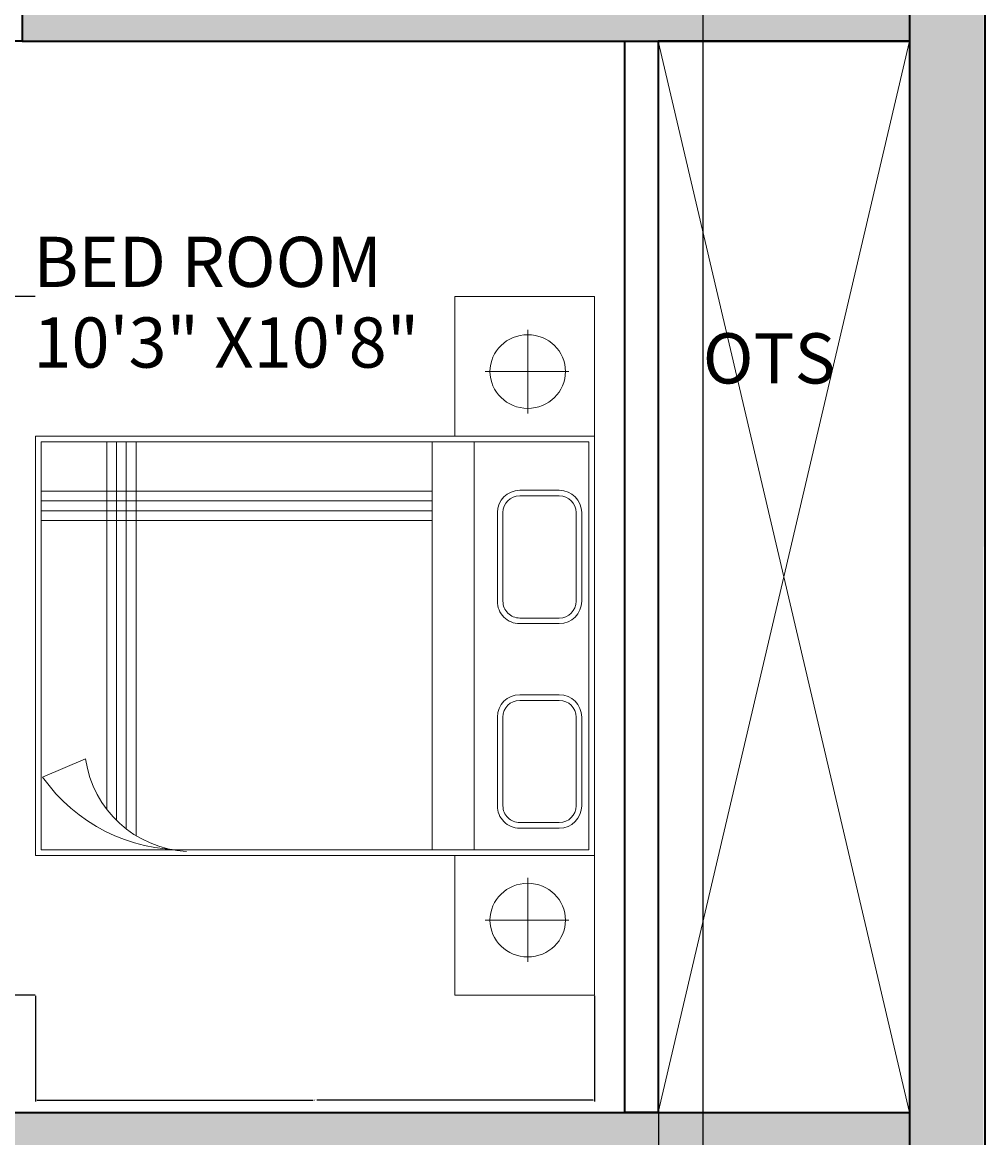
# Model space of a CAD drawing. Units: inches. Extents: x 2070 to 4408, y 1595 to 4269.
# Tile 16 of 20: x 2340 to 2455, y 1949 to 2083. Entities that reach past the tile are written whole.
import ezdxf

# ---------------------------------------------------------------- set-up
doc = ezdxf.new("R2010")
doc.units = ezdxf.units.IN
for name, color, linetype, lineweight in [('A-ANNO-DIMS', 2, 'Continuous', 18), ('A-AREA-IDEN', 7, 'Continuous', 18), ('A-FLOR-OPEN', 8, 'Continuous', 13), ('A-FURN', 8, 'Continuous', 18), ('A-WALL', 7, 'Continuous', 35)]:
    doc.layers.add(name, color=color, linetype=linetype, lineweight=lineweight)
doc.layers.add('A-WALL-PATT', color=18, linetype='Continuous', lineweight=13, true_color=0x000000)
doc.styles.get("Standard").update_dxf_attribs({"font": 'arial.ttf'})
doc.dimstyles.get("Standard").update_dxf_attribs({"dimtxt": 0.18, "dimasz": 0.18, "dimexe": 0.18, "dimexo": 0.0625, "dimgap": 0.09, "dimtad": 0, "dimtih": 1, "dimtoh": 1, "dimdec": 4, "dimzin": 0, "dimdsep": 46, "dimtxsty": 'Standard', "dimcen": 0.09, "dimadec": 0, "dimazin": 0, "dimtfac": 1, "dimtdec": 4, "dimtofl": 0, "dimtmove": 0, "dimatfit": 3, "dimfxl": 1, "dimtolj": 1, "dimtzin": 0, "dimarcsym": 0})

# ---------------------------------------------------------------- blocks, each defined once
blk = doc.blocks.new('A$C057D194F')
for p, q in [((0, 1.5, -0.1688), (0, 2, -0.1688)), ((0, 2, -0.1688), (0.5, 2, -0.1688)), ((0.5, 2, -0.1688), (0.5, 0, -0.1688)), ((2, 2, -0.1688), (0.5, 2, -0.1688)), ((2, 0, -0.1688), (2, 2, -0.1688)), ((2.5, 2, -0.1688), (2, 2, -0.1688)), ((2.5, 1.5, -0.1688), (2.5, 2, -0.1688)), ((1.98, 1.98, -0.1688), (0.52, 1.98, -0.1688)), ((0.52, 1.98, -0.1688), (0.52, 0.02, -0.1688)), ((1.98, 0.02, -0.1688), (1.98, 1.98, -0.1688)), ((1.0907, 1.9539, -0.1688), (0.7735, 1.9539, -0.1688)), ((1.0907, 1.9339, -0.1688), (0.7735, 1.9339, -0.1688)), ((1.8224, 1.9539, -0.1688), (1.5052, 1.9539, -0.1688)), ((1.8224, 1.9339, -0.1688), (1.5052, 1.9339, -0.1688)), ((0.2687, 1.9081, -0.1688), (0.2687, 1.761, -0.1688)), ((0.2687, 1.6081, -0.1688), (0.2687, 1.9081, -0.1688)), ((2.2313, 1.9081, -0.1688), (2.2313, 1.761, -0.1688)), ((2.2313, 1.6081, -0.1688), (2.2313, 1.9081, -0.1688)), ((0.6935, 1.8739, -0.1688), (0.6935, 1.7322, -0.1688)), ((0.7135, 1.8739, -0.1688), (0.7135, 1.7322, -0.1688)), ((1.1507, 1.7322, -0.1688), (1.1507, 1.8739, -0.1688)), ((1.1707, 1.7322, -0.1688), (1.1707, 1.8739, -0.1688)), ((1.4252, 1.8739, -0.1688), (1.4252, 1.7322, -0.1688)), ((1.4452, 1.8739, -0.1688), (1.4452, 1.7322, -0.1688)), ((1.8824, 1.7322, -0.1688), (1.8824, 1.8739, -0.1688)), ((1.9024, 1.7322, -0.1688), (1.9024, 1.8739, -0.1688)), ((0.4194, 1.761, -0.1688), (0.1194, 1.761, -0.1688)), ((0.2687, 1.761, -0.1688), (0.4194, 1.761, -0.1688)), ((0.2687, 1.761, -0.1688), (0.2687, 1.6081, -0.1688)), ((2.0806, 1.761, -0.1688), (2.3806, 1.761, -0.1688)), ((2.2313, 1.761, -0.1688), (2.0806, 1.761, -0.1688)), ((2.2313, 1.761, -0.1688), (2.2313, 1.6081, -0.1688)), ((0.7735, 1.6722, -0.1688), (1.0907, 1.6722, -0.1688)), ((0.7735, 1.6522, -0.1688), (1.0907, 1.6522, -0.1688)), ((1.5052, 1.6722, -0.1688), (1.8224, 1.6722, -0.1688)), ((1.5052, 1.6522, -0.1688), (1.8224, 1.6522, -0.1688)), ((1.98, 1.5693, -0.1688), (0.52, 1.5693, -0.1688)), ((0.5, 1.5, -0.1688), (0, 1.5, -0.1688)), ((2, 1.5, -0.1688), (2.5, 1.5, -0.1688)), ((1.98, 1.4193, -0.1688), (0.52, 1.4193, -0.1688)), ((0.6969, 0.02, -0.1688), (0.6969, 1.4193, -0.1688)), ((0.7319, 0.02, -0.1688), (0.7319, 1.4193, -0.1688)), ((0.7669, 0.02, -0.1688), (0.7669, 1.4193, -0.1688)), ((0.8019, 0.02, -0.1688), (0.8019, 1.4193, -0.1688)), ((0.52, 0.3595, -0.1688), (1.9292, 0.3595, -0.1688)), ((0.52, 0.3245, -0.1688), (1.905, 0.3245, -0.1688)), ((0.52, 0.2895, -0.1688), (1.8742, 0.2895, -0.1688)), ((0.52, 0.2545, -0.1688), (1.8344, 0.2545, -0.1688)), ((1.6548, 0.1789, -0.1688), (1.7198, 0.0251, -0.1688)), ((0.52, 0.02, -0.1688), (1.98, 0.02, -0.1688)), ((0.5, 0, -0.1688), (2, 0, -0.1688))]:
    blk.add_line(p, q)
for centre, radius, start, end in [((0.7735, 1.8739, -0.1688), 0.08, 90, 180), ((0.7735, 1.8739, -0.1688), 0.06, 90, 180), ((1.0907, 1.8739, -0.1688), 0.08, 0, 90), ((1.0907, 1.8739, -0.1688), 0.06, 0, 90), ((1.5052, 1.8739, -0.1688), 0.08, 90, 180), ((1.5052, 1.8739, -0.1688), 0.06, 90, 180), ((1.8224, 1.8739, -0.1688), 0.08, 0, 90), ((1.8224, 1.8739, -0.1688), 0.06, 0, 90), ((0.7735, 1.7322, -0.1688), 0.08, 180, 270), ((0.7735, 1.7322, -0.1688), 0.06, 180, 270), ((1.0907, 1.7322, -0.1688), 0.08, 270, 0), ((1.0907, 1.7322, -0.1688), 0.06, 270, 0), ((1.5052, 1.7322, -0.1688), 0.08, 180, 270), ((1.5052, 1.7322, -0.1688), 0.06, 180, 270), ((1.8224, 1.7322, -0.1688), 0.08, 270, 0), ((1.8224, 1.7322, -0.1688), 0.06, 270, 0), ((1.5992, 0.5623, -0.1688), 0.3874, 278.2518, 356.6808), ((1.363, 0.5286, -0.1688), 0.6171, 305.3295, 1.0459)]:
    blk.add_arc(centre, radius, start, end)
blk.add_ellipse((0.2687, 1.761, -0.1688), major_axis=(0, -0.1351), ratio=0.975448)
at = {"extrusion": (0, 0, -1)}
blk.add_ellipse((2.2313, 1.761, -0.1688), major_axis=(0, 0.1351), ratio=0.975448, dxfattribs=at)
for p in [(0.2687, 1.761, -0.1688), (2.2313, 1.761, -0.1688)]:
    blk.add_point(p)
blk = doc.blocks.new('*D15')
at = {"layer": 'A-ANNO-DIMS', "color": 0, "lineweight": -2, "transparency": 16777216}
for p, q in [((2341.72, 2049.92), (2329.08, 2049.92)), ((2329.26, 2049.74), (2329.26, 2008.35)), ((2329.26, 1966.6), (2329.26, 2007.99)), ((2341.72, 1966.42), (2329.08, 1966.42))]:
    blk.add_line(p, q, dxfattribs=at)
at = {"layer": 'A-ANNO-DIMS', "color": 0, "transparency": 16777216}
for points in [[(2329.23, 2049.74), (2329.29, 2049.74), (2329.26, 2049.92)], [(2329.23, 1966.6), (2329.29, 1966.6), (2329.26, 1966.42)]]:
    blk.add_solid(points, dxfattribs=at)
at = {"layer": 'Defpoints', "color": 0, "transparency": 16777216}
for p in [(2341.78, 2049.92), (2329.26, 1966.42), (2341.78, 1966.42)]:
    blk.add_point(p, dxfattribs=at)
at = {"layer": 'A-ANNO-DIMS', "color": 0, "transparency": 16777216, "insert": (2329.26, 2008.17), "char_height": 0.18, "attachment_point": 5}
blk.add_mtext('\\A1;BED SET 83', dxfattribs=at)
blk = doc.blocks.new('*D16')
at = {"layer": 'A-ANNO-DIMS', "color": 0, "lineweight": -2, "transparency": 16777216}
for p, q in [((2341.78, 1966.36), (2341.78, 1953.72)), ((2408.58, 1966.36), (2408.58, 1953.72)), ((2341.96, 1953.9), (2374.96, 1953.9)), ((2408.4, 1953.9), (2375.4, 1953.9))]:
    blk.add_line(p, q, dxfattribs=at)
at = {"layer": 'A-ANNO-DIMS', "color": 0, "transparency": 16777216}
for points in [[(2341.96, 1953.93), (2341.96, 1953.87), (2341.78, 1953.9)], [(2408.4, 1953.93), (2408.4, 1953.87), (2408.58, 1953.9)]]:
    blk.add_solid(points, dxfattribs=at)
at = {"layer": 'Defpoints', "color": 0, "transparency": 16777216}
for p in [(2341.78, 1966.42), (2408.58, 1966.42), (2408.58, 1953.9)]:
    blk.add_point(p, dxfattribs=at)
at = {"layer": 'A-ANNO-DIMS', "color": 0, "transparency": 16777216, "insert": (2375.18, 1953.9), "char_height": 0.18, "attachment_point": 5}
blk.add_mtext('\\A1;67', dxfattribs=at)
blk = doc.blocks.new('*D30')
at = {"layer": 'A-ANNO-DIMS', "color": 0, "lineweight": -2, "transparency": 16777216}
for p, q in [((2416.2, 2080.34), (2416.2, 1595.04)), ((2446.2, 2080.34), (2446.2, 1595.04)), ((2416.38, 1595.22), (2430.98, 1595.22)), ((2446.02, 1595.22), (2431.41, 1595.22))]:
    blk.add_line(p, q, dxfattribs=at)
at = {"layer": 'A-ANNO-DIMS', "color": 0, "transparency": 16777216}
for points in [[(2416.38, 1595.25), (2416.38, 1595.19), (2416.2, 1595.22)], [(2446.02, 1595.25), (2446.02, 1595.19), (2446.2, 1595.22)]]:
    blk.add_solid(points, dxfattribs=at)
at = {"layer": 'Defpoints', "color": 0, "transparency": 16777216}
for p in [(2416.2, 2080.4), (2446.2, 2080.4), (2446.2, 1595.22)]:
    blk.add_point(p, dxfattribs=at)
at = {"layer": 'A-ANNO-DIMS', "color": 0, "transparency": 16777216, "insert": (2431.2, 1595.22), "char_height": 0.18, "attachment_point": 5}
blk.add_mtext('\\A1;30', dxfattribs=at)
blk = doc.blocks.new('*D34')
at = {"layer": 'A-ANNO-DIMS', "color": 0, "lineweight": -2, "transparency": 16777216}
for p, q in [((2421.53, 2212.34), (2421.53, 1595.04)), ((2446.2, 2212.34), (2446.2, 1595.04)), ((2421.71, 1595.22), (2433.4, 1595.22)), ((2446.02, 1595.22), (2434.33, 1595.22))]:
    blk.add_line(p, q, dxfattribs=at)
at = {"layer": 'A-ANNO-DIMS', "color": 0, "transparency": 16777216}
for points in [[(2421.71, 1595.25), (2421.71, 1595.19), (2421.53, 1595.22)], [(2446.02, 1595.25), (2446.02, 1595.19), (2446.2, 1595.22)]]:
    blk.add_solid(points, dxfattribs=at)
at = {"layer": 'Defpoints', "color": 0, "transparency": 16777216}
for p in [(2421.53, 2212.4), (2446.2, 2212.4), (2446.2, 1595.22)]:
    blk.add_point(p, dxfattribs=at)
at = {"layer": 'A-ANNO-DIMS', "color": 0, "transparency": 16777216, "insert": (2433.86, 1595.22), "char_height": 0.18, "attachment_point": 5}
blk.add_mtext('\\A1;24.663', dxfattribs=at)

msp = doc.modelspace()

# ---------------------------------------------------------------- hatches: boundary and pattern name
at = {"layer": 'A-WALL-PATT'}
h = msp.add_hatch(color=256, dxfattribs=at)
h.dxf.hatch_style = 1
h.paths.add_polyline_path([(2346.196, 2218.3995), (2346.196, 2282.3995), (2340.196, 2282.3995), (2340.196, 2212.3995), (2345.5866, 2212.3995), (2346.196, 2212.3995)], flags=0)
h.paths.add_polyline_path([(2245.196, 2282.3995), (2239.196, 2282.3995), (2239.196, 2186.3995), (2244.5866, 2186.3995), (2245.196, 2186.3995)], flags=0)
h.paths.add_polyline_path([(2340.196, 2230.6455), (2245.196, 2230.6455), (2245.196, 2224.6455), (2340.196, 2224.6455)], flags=0)
h.paths.add_polyline_path([(2245.196, 2150.3995), (2239.196, 2150.3995), (2164.4362, 2150.3995), (2164.4362, 2144.3995), (2239.196, 2144.3995), (2239.196, 2086.3995), (2239.196, 2067.2711), (2244.5866, 2067.2711), (2245.196, 2067.2711), (2245.196, 2144.3995)], flags=0)
h.paths.add_polyline_path([(2346.196, 2176.3995), (2340.196, 2176.3995), (2340.196, 2086.3995), (2346.196, 2086.3995), (2346.196, 2125.318)], flags=0)
h.paths.add_polyline_path([(2446.196, 2086.3995), (2346.196, 2086.3995), (2340.196, 2086.3995), (2340.196, 2080.3995), (2446.196, 2080.3995)], flags=0)
h.paths.add_polyline_path([(2455.196, 2291.3995), (2103.196, 2291.3995), (2103.196, 1699.3995), (2336.196, 1699.3995), (2336.196, 1628.3995), (2345.196, 1628.3995), (2446.196, 1628.3995), (2454.8846, 1628.3995), (2454.8846, 1699.3995)])
h.paths.add_polyline_path([(2446.196, 2282.3995), (2446.196, 2218.3995), (2446.196, 2212.3995), (2446.196, 2086.3995), (2446.196, 2080.3995), (2446.196, 1708.3995), (2446.196, 1637.3995), (2345.196, 1637.3995), (2345.196, 1699.3995), (2345.196, 1708.3995), (2336.196, 1708.3995), (2112.196, 1708.3995), (2112.196, 2282.3995), (2239.196, 2282.3995), (2245.196, 2282.3995), (2356.196, 2282.3995)], flags=16)
h.paths.add_polyline_path([(2245.196, 2150.3995), (2245.196, 2144.3995), (2245.196, 2067.2711), (2244.5866, 2067.2711), (2239.196, 2067.2711), (2239.196, 2065.6988), (2203.2929, 2065.6988, 0.40145271), (2239.196, 2031.3337), (2244.5866, 2031.3337), (2245.196, 2031.2711), (2245.196, 1924.1525), (2239.196, 1924.1525), (2239.196, 1922.5803), (2203.2929, 1922.5803, 0.40145271), (2239.196, 1888.2151), (2244.5866, 1888.2151), (2245.196, 1888.1525), (2245.196, 1748.3995), (2339.196, 1748.4621, -0.40145271), (2303.2929, 1782.8272), (2303.2585, 1782.8272), (2303.2585, 1784.3995), (2339.196, 1784.3995), (2339.196, 1877.2067), (2291.196, 1877.2067), (2291.196, 1883.2067), (2291.196, 1946.3995), (2291.196, 1952.3995), (2291.196, 2086.3995), (2297.196, 2086.3995), (2302.196, 2086.3995), (2302.196, 2081.0259), (2303.7633, 2081.0259), (2303.7633, 2080.3995), (2338.0148, 2080.3995, 0.00437129), (2338.0203, 2081.0259), (2338.0203, 2086.3995), (2340.196, 2086.3995), (2340.196, 2176.4621), (2345.5866, 2176.4621, 0.40145271), (2381.4896, 2210.8272), (2345.5866, 2210.8272), (2345.5866, 2212.3995), (2340.196, 2212.3995), (2340.196, 2224.6455), (2245.196, 2224.6455), (2245.196, 2186.3995), (2244.5866, 2186.3995), (2239.196, 2186.3995), (2239.196, 2184.8272), (2203.2929, 2184.8272, 0.40145271), (2239.196, 2150.4621), (2244.5866, 2150.4621)], flags=0)
h.paths.add_polyline_path([(2346.196, 2282.3995), (2346.196, 2218.3995), (2377.1813, 2218.3995), (2377.1813, 2212.3995), (2346.196, 2212.3995), (2345.5866, 2212.3995), (2340.196, 2212.3995), (2340.196, 2224.6455), (2245.196, 2224.6455), (2245.196, 2230.6455), (2245.196, 2282.3995), (2292.696, 2256.5225), (2340.196, 2282.3995)], flags=0)
h.paths.add_polyline_path([(2346.196, 2086.3995), (2340.196, 2086.3995), (2340.196, 2080.3995), (2446.196, 2080.3995), (2431.196, 2016.3995), (2446.196, 1952.3995), (2412.196, 1952.3995), (2412.196, 2080.3995), (2340.196, 2080.3995), (2340.196, 2086.3995), (2340.196, 2176.3995), (2346.196, 2176.3995), (2346.196, 2125.318)], flags=0)
h.paths.add_polyline_path([(2186.508, 2270.0471, -0.03755288), (2186.9712, 2269.8581), (2186.9164, 2270.112, -0.02759121)], flags=0)
h.paths.add_polyline_path([(2183.955, 2273.7766, 1), (2188.2945, 2273.7766, 1)], flags=0)
h.paths.add_polyline_path([(2142.5261, 2274.6158, -0.03707541), (2142.5672, 2275.1696), (2142.5672, 2276.826), (2119.8759, 2276.826), (2119.8759, 2263.0962), (2140.4332, 2263.0962), (2142.5672, 2263.0962), (2142.5672, 2274.0621, -0.03707541)], flags=0)
h.paths.add_polyline_path([(2209.8974, 2263.0962), (2209.8974, 2262.2079), (2190.8042, 2262.2079), (2190.8042, 2263.0962)], flags=0)
h.paths.add_polyline_path([(2210.6382, 2276.1833), (2210.6382, 2263.9844), (2190.2185, 2263.9844), (2190.2185, 2276.1833)], flags=0)
h.paths.add_polyline_path([(2188.4362, 2273.7766, -1), (2183.8133, 2273.7766, -1)], flags=0)
h.paths.add_polyline_path([(2245.196, 2150.3995), (2245.196, 2144.3995), (2245.196, 2067.2711), (2239.196, 2067.2711), (2239.196, 2080.3995), (2172.196, 2080.3995), (2172.196, 2000.3995), (2239.196, 2000.3995), (2239.196, 1940.3995), (2159.0187, 1940.3995), (2123.0187, 1940.3995), (2112.196, 1940.3995), (2112.196, 1946.3995), (2123.0187, 1946.3995), (2123.0187, 1982.2238), (2124.586, 1982.2238), (2124.586, 1982.1895, -0.40145271), (2158.8429, 1946.3995), (2159.0187, 1946.3995), (2239.196, 1946.3995), (2239.196, 1994.3995), (2112.196, 1994.3995), (2112.196, 2000.3995), (2139.196, 2040.3995), (2112.196, 2080.3995), (2112.196, 2086.3995), (2239.196, 2086.3995), (2239.196, 2144.3995), (2209.5809, 2144.3995), (2209.5809, 2136.3995), (2203.0809, 2136.3995), (2205.0809, 2130.3996, -0.70257121), (2199.081, 2116.3995, -0.70256205), (2193.0809, 2130.3994), (2195.0809, 2136.3995), (2192.0809, 2136.3995), (2192.0809, 2134.8995), (2189.0809, 2134.8995), (2189.0809, 2135.8995), (2191.0809, 2135.8995), (2191.0809, 2136.3995), (2188.5809, 2136.3995), (2188.5809, 2144.3995), (2164.2481, 2144.3995, -0.39385849), (2130.0035, 2109.5491), (2130.0035, 2109.5147), (2128.4362, 2109.5147), (2128.4362, 2144.3995), (2112.196, 2144.3995), (2112.196, 2150.3995), (2128.4362, 2150.3995), (2128.4362, 2150.7127), (2164.4362, 2150.7127), (2164.4362, 2150.3995), (2239.196, 2150.3995)], flags=0)
h.paths.add_polyline_path([(2188.2075, 2266.8735), (2188.2075, 2211.8632, -0.41421356), (2185.4833, 2209.1391), (2146.7995, 2209.1391, -0.41421356), (2144.0754, 2211.8632), (2144.0754, 2266.8735, -0.41421356), (2146.7995, 2269.5976), (2185.4833, 2269.5976, -0.41421356)], flags=0)
h.paths.add_polyline_path([(2185.0844, 2273.7766, -1), (2187.1651, 2273.7766, -1)], flags=0)
h.paths.add_polyline_path([(2182.0486, 2259.2932), (2168.0953, 2259.2932), (2168.0953, 2260.8424), (2163.7261, 2260.8424), (2163.7261, 2259.2932), (2149.7727, 2259.2932), (2149.7727, 2266.3352), (2163.7261, 2266.3352), (2163.7261, 2261.9839), (2168.0953, 2261.9839), (2168.0953, 2266.3352), (2182.0486, 2266.3352)], flags=0)
h.paths.add_polyline_path([(2148.2585, 2250.2051), (2153.0615, 2241.8861, 0.39807048)], flags=0)
h.paths.add_polyline_path([(2162.7572, 2247.2885), (2153.1461, 2241.7396), (2148.1083, 2250.4653), (2157.7194, 2256.0142)], flags=0)
h.paths.add_polyline_path([(2162.6726, 2247.4351, -0.39286196), (2157.8415, 2255.6313), (2157.6431, 2255.6313), (2157.8696, 2255.7541)], flags=0)
h.paths.add_polyline_path([(2164.2604, 2145.339), (2164.4362, 2144.3995), (2164.4362, 2150.3995), (2164.2604, 2150.7127)], flags=0)
h.paths.add_polyline_path([(2208.5809, 2142.6495), (2208.5809, 2138.3995, -0.41421356), (2207.8309, 2137.3995), (2190.5809, 2137.3995, -0.41421356), (2189.5809, 2138.1495), (2189.5809, 2142.3995, -0.41421356), (2190.3309, 2143.3995), (2207.5809, 2143.3995, -0.41421356)], flags=0)
h.paths.add_polyline_path([(2147.957, 2229.9119), (2154.7494, 2223.1195, 0.39807048)], flags=0)
h.paths.add_polyline_path([(2162.7165, 2230.8473), (2154.8691, 2222.9998), (2147.7446, 2230.1244), (2155.592, 2237.9718)], flags=0)
h.paths.add_polyline_path([(2162.5969, 2230.9669, -0.39807048), (2155.8044, 2237.7594)], flags=0)
h.paths.add_polyline_path([(2391.8776, 2049.9192), (2408.5766, 2049.9192), (2408.5766, 2033.2202), (2408.5766, 1983.123), (2408.5766, 1966.4239), (2391.8776, 1966.4239), (2391.8776, 1983.123), (2341.7804, 1983.123), (2341.7804, 2033.2202), (2391.8776, 2033.2202)], flags=0)
h.paths.add_polyline_path([(2144.1055, 2274.6158, 1), (2148.445, 2274.6158, 1)], flags=0)
h.paths.add_polyline_path([(2148.5867, 2274.6158, -1), (2143.9638, 2274.6158, -1)], flags=0)
h.paths.add_polyline_path([(2145.2349, 2274.6158, -1), (2147.3156, 2274.6158, -1)], flags=0)
edge = h.paths.add_edge_path(flags=0)
edge.add_ellipse((2400.5951, 2040.9436), major_axis=(-4.5109, 0), ratio=0.97544784, start_angle=180, end_angle=270, ccw=False)
edge.add_ellipse((2400.5951, 2040.9436), major_axis=(-4.5109, 0), ratio=0.97544784, start_angle=90, end_angle=180, ccw=False)
edge.add_ellipse((2400.5951, 2040.9436), major_axis=(-4.5109, 0), ratio=0.97544784, start_angle=0, end_angle=90, ccw=False)
edge.add_ellipse((2400.5951, 2040.9436), major_axis=(-4.5109, 0), ratio=0.97544784, start_angle=270, end_angle=360, ccw=False)
h.paths.add_polyline_path([(2199.0809, 2117.3995, -0.73452973), (2195.0809, 2130.3995), (2203.081, 2130.3995, -0.73453329)], flags=0)
h.paths.add_polyline_path([(2141.9147, 2276.0353), (2141.9147, 2263.9844), (2120.4685, 2263.9844), (2120.4685, 2276.0353)], flags=0)
h.paths.add_polyline_path([(2138.4481, 2273.4072), (2138.4481, 2266.7226), (2133.2801, 2266.7226), (2133.2801, 2273.4072)], flags=0)
h.paths.add_polyline_path([(2137.9691, 2272.9175), (2137.9691, 2272.204), (2135.4229, 2272.204), (2135.4229, 2271.6329), (2135.3221, 2270.1051), (2135.3221, 2269.0265), (2135.4229, 2268.6811), (2135.4229, 2267.2011), (2133.7212, 2267.2011), (2133.7212, 2268.6811), (2133.7983, 2269.9587), (2133.7983, 2271.2758), (2133.7212, 2271.6329), (2133.7212, 2273.0065), (2135.717, 2273.0065), (2135.717, 2272.9175)], flags=0)
h.paths.add_polyline_path([(2137.9215, 2271.8264), (2137.9215, 2271.3786), (2137.5182, 2271.3786), (2136.9355, 2271.3786), (2136.3529, 2271.3786), (2135.7703, 2271.3786), (2135.7703, 2271.8264), (2136.1736, 2271.8264), (2136.7562, 2271.8264), (2137.3389, 2271.8264)], flags=0)
h.paths.add_polyline_path([(2137.9215, 2271.692), (2137.5182, 2271.692), (2136.9355, 2271.513), (2137.3389, 2271.513)], flags=0)
h.paths.add_polyline_path([(2136.3529, 2271.692), (2135.7703, 2271.513), (2136.1736, 2271.513), (2136.7562, 2271.692)], flags=0)
h.paths.add_polyline_path([(2137.9215, 2271.513), (2137.5182, 2271.513), (2136.7562, 2271.747), (2136.7562, 2271.692), (2137.3389, 2271.692)], flags=0)
h.paths.add_polyline_path([(2137.8207, 2270.4664), (2137.8207, 2270.0971), (2137.8207, 2269.627), (2137.8207, 2269.1569), (2137.8207, 2268.6868), (2137.3837, 2268.6868), (2136.6442, 2268.6868), (2135.9271, 2268.6868), (2135.9271, 2269.0562), (2135.9271, 2269.5263), (2135.9271, 2269.9963), (2135.9271, 2270.4664), (2136.3641, 2270.4664), (2137.0812, 2270.4664)], flags=0)
h.paths.add_polyline_path([(2137.3837, 2269.627), (2137.8207, 2269.627), (2137.8207, 2269.5263), (2137.3837, 2269.5263), (2137.3837, 2269.1569), (2137.8207, 2269.1569), (2137.3837, 2269.0562), (2137.3837, 2268.6868), (2137.0812, 2268.6868), (2137.0812, 2269.0562), (2136.6442, 2269.0562), (2136.6442, 2268.6868), (2136.3641, 2268.6868), (2136.3641, 2269.0562), (2135.9271, 2269.0562), (2135.9271, 2269.1569), (2136.3641, 2269.1569), (2136.3641, 2269.5263), (2135.9271, 2269.5263), (2135.9271, 2269.627), (2136.3641, 2269.627), (2136.3641, 2269.9963), (2135.9271, 2269.9963), (2136.3641, 2270.0971), (2136.3641, 2270.4664), (2136.6442, 2270.4664), (2136.6442, 2270.0971), (2137.0812, 2270.0971), (2137.0812, 2270.4664), (2137.3837, 2270.4664), (2137.3837, 2270.0971), (2137.8207, 2270.0971), (2137.3837, 2269.9963)], flags=0)
h.paths.add_polyline_path([(2137.5182, 2271.8264), (2137.5182, 2271.692), (2137.3389, 2271.3786), (2137.3389, 2271.513)], flags=0)
h.paths.add_polyline_path([(2137.8179, 2267.8138), (2137.8179, 2267.6879), (2137.1876, 2267.6879), (2136.4733, 2267.6879), (2135.759, 2267.6879), (2135.759, 2267.8138), (2136.3893, 2267.8138), (2137.1036, 2267.8138)], flags=0)
h.paths.add_polyline_path([(2137.0812, 2269.9963), (2137.0812, 2269.627), (2137.0812, 2269.1569), (2136.6442, 2269.1569), (2136.6442, 2269.5263), (2136.6442, 2269.9963)], flags=0)
h.paths.add_polyline_path([(2136.3529, 2271.8264), (2136.3529, 2271.692), (2136.1736, 2271.3786), (2136.1736, 2271.513)], flags=0)
h.paths.add_polyline_path([(2136.4733, 2267.8138), (2136.4733, 2267.6879), (2136.3893, 2267.6879), (2136.3893, 2267.8138)], flags=0)
h.paths.add_polyline_path([(2407.9087, 2032.5522), (2407.9087, 1983.7909), (2359.81, 1983.7909, -0.00912788), (2359.0575, 1983.7909), (2342.4483, 1983.7909), (2342.4483, 2032.5522)], flags=0)
h.paths.add_polyline_path([(2389.1838, 2023.1358), (2353.7856, 2023.1358), (2353.7856, 1985.4867, -0.09210376), (2350.2788, 1988.655), (2350.2788, 2026.6426), (2389.1838, 2026.6426)], flags=0)
h.paths.add_polyline_path([(2352.6166, 2024.3048), (2351.4477, 2024.3048), (2351.4477, 2025.4737), (2352.6166, 2025.4737)], flags=0)
h.paths.add_polyline_path([(2399.6319, 2026.7589), (2404.3661, 2026.7589, -0.41421356), (2407.0379, 2024.087), (2407.0379, 2013.4908, -0.41421356), (2404.3661, 2010.819), (2399.6319, 2010.819, -0.41421356), (2396.96, 2013.4908), (2396.96, 2024.087, -0.41421356)], flags=0)
h.paths.add_polyline_path([(2399.6319, 2026.0909), (2404.3661, 2026.0909, -0.41421356), (2406.37, 2024.087), (2406.37, 2013.4908, -0.41421356), (2404.3661, 2011.487), (2399.6319, 2011.487, -0.41421356), (2397.628, 2013.4908), (2397.628, 2024.087, -0.41421356)], flags=0)
h.paths.add_polyline_path([(2399.6319, 2002.3217), (2404.3661, 2002.3217, -0.41421356), (2407.0379, 1999.6498), (2407.0379, 1989.0536, -0.41421356), (2404.3661, 1986.3818), (2399.6319, 1986.3818, -0.41421356), (2396.96, 1989.0536), (2396.96, 1999.6498, -0.41421356)], flags=0)
h.paths.add_polyline_path([(2399.6319, 2001.6537), (2404.3661, 2001.6537, -0.41421356), (2406.37, 1999.6498), (2406.37, 1989.0536, -0.41421356), (2404.3661, 1987.0497), (2399.6319, 1987.0497, -0.41421356), (2397.628, 1989.0536), (2397.628, 1999.6498, -0.41421356)], flags=0)
edge = h.paths.add_edge_path(flags=0)
edge.add_ellipse((2400.5951, 1975.3996), major_axis=(-4.5109, 0), ratio=0.97544784, start_angle=-180, end_angle=-90, ccw=False)
edge.add_ellipse((2400.5951, 1975.3996), major_axis=(-4.5109, 0), ratio=0.97544784, start_angle=90, end_angle=180, ccw=False)
edge.add_ellipse((2400.5951, 1975.3996), major_axis=(-4.5109, 0), ratio=0.97544784, start_angle=0, end_angle=90, ccw=False)
edge.add_ellipse((2400.5951, 1975.3996), major_axis=(-4.5109, 0), ratio=0.97544784, start_angle=-90, end_angle=0, ccw=False)
h.paths.add_polyline_path([(2345.196, 1910.3995), (2366.4386, 1910.3995), (2366.4386, 1925.4555), (2392.3856, 1925.4555), (2392.3856, 1933.5025), (2400.1399, 1925.4555), (2392.3856, 1919.8795), (2392.3856, 1925.4555), (2366.4386, 1925.4555), (2366.4386, 1910.3995), (2381.196, 1910.3995), (2405.196, 1910.3995), (2405.196, 1898.3995), (2446.196, 1898.3995), (2446.196, 1886.3995), (2405.196, 1886.3995), (2405.196, 1874.3995), (2446.196, 1874.3995), (2446.196, 1862.3995), (2405.196, 1862.3995), (2405.196, 1850.3995), (2446.196, 1850.3995), (2446.196, 1838.3995), (2405.196, 1838.3995), (2405.196, 1826.3995), (2446.196, 1826.3995), (2446.196, 1814.3995), (2405.196, 1814.3995), (2405.196, 1802.3995), (2446.196, 1802.3995), (2446.196, 1798.3995), (2446.196, 1792.3995), (2405.196, 1792.3995), (2405.196, 1910.3995), (2381.196, 1910.3995), (2381.196, 1792.3995), (2345.196, 1792.3995)], flags=0)
h.paths.add_polyline_path([(2333.0944, 1863.3993, -0.41421356), (2334.7225, 1861.7712), (2334.7225, 1859.329), (2335.2653, 1859.329, -0.41421356), (2337.4361, 1857.1582), (2337.4361, 1843.862, -0.41421356), (2335.2653, 1841.6911, -0.41421356), (2337.4361, 1839.5203), (2337.4361, 1827.5808, -0.41421356), (2335.2653, 1825.41, -0.41421356), (2337.4361, 1823.2392), (2337.4361, 1808.5862, -0.41421356), (2335.2653, 1806.4153), (2334.7225, 1806.4153), (2334.7225, 1803.9732, -0.41421356), (2333.0944, 1802.3451), (2317.356, 1802.3451), (2317.0846, 1802.3451, -0.41421356), (2315.7279, 1803.7018), (2315.7279, 1803.8646), (2313.8284, 1803.8646, -0.41421356), (2311.6576, 1806.0354), (2311.6576, 1823.2015, -0.39597602), (2313.6834, 1825.3765, -0.43384798), (2311.6576, 1827.2718), (2311.6576, 1839.761, -0.41421356), (2313.5571, 1841.6604), (2313.8284, 1841.6604), (2333.8159, 1841.6604, -0.04213623), (2334.1798, 1841.6911, -0.41421356), (2332.009, 1843.862), (2332.009, 1857.1582, -0.41421356), (2334.1798, 1859.329), (2317.356, 1859.329), (2317.0846, 1859.329, -0.41421356), (2315.7279, 1860.6858), (2315.7279, 1862.0426, -0.41421356), (2317.0846, 1863.3993), (2317.356, 1863.3993)], flags=0)
h.paths.add_polyline_path([(2208.8475, 1848.9818), (2208.8475, 1840.9741, -0.41421356), (2207.0458, 1839.1724), (2206.5453, 1839.1721), (2206.5453, 1838.7218, -0.40985861), (2204.7704, 1836.9203), (2183.7501, 1836.9203, -0.41858196), (2181.9216, 1838.7218), (2181.9216, 1839.1721), (2181.421, 1839.1724, -0.41421356), (2179.6193, 1840.9741), (2179.6193, 1848.6817, -0.44064415), (2185.1126, 1854.9874), (2203.3852, 1854.9874, -0.45707961)], flags=0)
h.paths.add_polyline_path([(2204.243, 1848.4815), (2204.243, 1848.4815, 0.41725335), (2202.2204, 1850.4833), (2186.2049, 1850.4833, 0.4111805), (2184.2237, 1848.4815), (2184.2237, 1848.4815, -0.4111807), (2186.2049, 1850.4833), (2202.2204, 1850.4833, -0.41725315)], flags=0)
h.paths.add_polyline_path([(2234.7177, 1830.228), (2234.7176, 1781.6047, -0.41421356), (2233.4381, 1780.3252), (2218.6064, 1780.3252, -0.41421356), (2217.8387, 1781.0929), (2217.8387, 1783.3961, -0.41421356), (2218.6064, 1784.1639), (2218.6065, 1796.9595, -0.41421356), (2219.886, 1798.239, -0.41421356), (2218.6065, 1799.5186), (2218.6065, 1812.3142, -0.41421356), (2219.8861, 1813.5938, -0.41421356), (2218.6065, 1814.8733), (2218.6065, 1827.6689, -0.41421356), (2217.8388, 1828.4367), (2217.8388, 1830.7399, -0.41421356), (2218.6065, 1831.5076), (2233.4382, 1831.5076, -0.41421356)], flags=0)
h.paths.add_polyline_path([(2230.6344, 1827.6689, -0.41421356), (2231.4021, 1826.9012), (2231.4021, 1784.9316, -0.41421356), (2230.6343, 1784.1639), (2221.1853, 1784.1639), (2221.1853, 1827.6689)], flags=0)
h.paths.add_polyline_path([(2222.7208, 1798.239), (2221.6971, 1798.239), (2221.6971, 1813.5938), (2222.7208, 1813.5938)], flags=0)
h.paths.add_polyline_path([(2206.5453, 1773.935), (2206.5453, 1773.4848), (2206.9457, 1773.4848), (2207.0458, 1773.4845, -0.41421356), (2208.8475, 1771.6827), (2208.8475, 1763.675, -0.44222432), (2203.6505, 1757.6695), (2185.3851, 1757.6695, -0.45508402), (2179.6193, 1763.9752), (2179.6193, 1771.6827, -0.41421356), (2181.421, 1773.4845), (2181.421, 1773.4848), (2181.9216, 1773.4848), (2181.9216, 1773.935, -0.40985861), (2183.6965, 1775.7366), (2204.7167, 1775.7366, -0.41858196)], flags=0)
h.paths.add_polyline_path([(2202.2619, 1762.1736), (2186.2464, 1762.1736, -0.41725315), (2184.2237, 1764.1754), (2184.2237, 1764.1754, 0.41725335), (2186.2464, 1762.1736), (2202.2619, 1762.1736, 0.4111805), (2204.243, 1764.1754), (2204.243, 1764.1754, -0.4111807)], flags=0)
h.paths.add_polyline_path([(2313.0034, 1713.1906), (2312.997, 1713.1697), (2313.0123, 1713.1612)], flags=0)
h.paths.add_polyline_path([(2305.7314, 1721.0488), (2305.6257, 1721.1994), (2305.4853, 1721.084)], flags=0)
h.paths.add_polyline_path([(2307.5562, 1726.1427), (2307.6186, 1726.1026), (2307.5737, 1726.0477), (2308.5692, 1720.6434), (2310.5345, 1721.2985), (2310.5721, 1721.411), (2310.6958, 1721.3523), (2313.8453, 1722.4021), (2314.9351, 1723.8033), (2314.9294, 1723.9165), (2315.0028, 1723.8903), (2313.874, 1722.4389), (2313.8697, 1722.4102), (2308.5692, 1720.6434), (2308.9864, 1720.122), (2309.0665, 1720.0971), (2309.053, 1720.0387), (2310.9235, 1717.7005), (2311.4182, 1717.6259), (2311.2918, 1717.2402), (2312.0655, 1716.2731), (2312.1081, 1716.2606), (2312.0969, 1716.2339), (2308.5692, 1720.6434), (2305.2249, 1717.745), (2305.232, 1717.704), (2305.1665, 1717.6944), (2308.5692, 1720.6434)], flags=0)
h.paths.add_polyline_path([(2288.2072, 1714.3431), (2288.2008, 1714.3222), (2288.216, 1714.3137)], flags=0)
h.paths.add_polyline_path([(2280.9352, 1722.2013), (2280.8295, 1722.3519), (2280.689, 1722.2365)], flags=0)
h.paths.add_polyline_path([(2282.76, 1727.2952), (2282.8224, 1727.2551), (2282.7775, 1727.2002), (2283.773, 1721.7959), (2285.7383, 1722.451), (2285.7759, 1722.5635), (2285.8995, 1722.5048), (2289.0491, 1723.5546), (2290.1389, 1724.9558), (2290.1332, 1725.069), (2290.2065, 1725.0428), (2289.0777, 1723.5915), (2289.0735, 1723.5628), (2283.773, 1721.7959), (2284.1901, 1721.2745), (2284.2703, 1721.2496), (2284.2567, 1721.1913), (2286.1273, 1718.8531), (2286.622, 1718.7785), (2286.4956, 1718.3927), (2287.2692, 1717.4256), (2287.3119, 1717.4131), (2287.3006, 1717.3864), (2283.773, 1721.7959), (2280.4286, 1718.8975), (2280.4357, 1718.8565), (2280.3703, 1718.8469), (2283.773, 1721.7959)], flags=0)
h.paths.add_polyline_path([(2302.0672, 1721.8694), (2301.8205, 1721.8572), (2301.7578, 1722.1787), (2299.415, 1724.5215), (2299.103, 1724.4694), (2299.0662, 1724.8703)], flags=0)
h.paths.add_polyline_path([(2264.5643, 1715.4956), (2264.5579, 1715.4747), (2264.5731, 1715.4662)], flags=0)
h.paths.add_polyline_path([(2257.2923, 1723.3538), (2257.1865, 1723.5044), (2257.0461, 1723.389)], flags=0)
h.paths.add_polyline_path([(2259.117, 1728.4477), (2259.1795, 1728.4077), (2259.1345, 1728.3527), (2260.13, 1722.9484), (2262.0954, 1723.6036), (2262.133, 1723.716), (2262.2566, 1723.6573), (2265.4061, 1724.7071), (2266.4959, 1726.1083), (2266.4902, 1726.2215), (2266.5636, 1726.1953), (2265.4348, 1724.744), (2265.4305, 1724.7153), (2260.13, 1722.9484), (2260.5472, 1722.427), (2260.6273, 1722.4022), (2260.6138, 1722.3438), (2262.4843, 1720.0056), (2262.979, 1719.931), (2262.8526, 1719.5452), (2263.6263, 1718.5781), (2263.6689, 1718.5656), (2263.6577, 1718.5389), (2260.13, 1722.9484), (2256.7857, 1720.05), (2256.7928, 1720.009), (2256.7273, 1719.9994), (2260.13, 1722.9484)], flags=0)
h.paths.add_polyline_path([(2277.2709, 1723.0219), (2277.0243, 1723.0097), (2276.9616, 1723.3312), (2274.6187, 1725.6741), (2274.3067, 1725.6219), (2274.27, 1726.0228)], flags=0)
h.paths.add_polyline_path([(2253.628, 1724.1744), (2253.3814, 1724.1622), (2253.3186, 1724.4838), (2250.9758, 1726.8266), (2250.6638, 1726.7744), (2250.627, 1727.1753)], flags=0)
h.paths.add_polyline_path([(2161.9194, 1715.4956), (2161.913, 1715.4747), (2161.9282, 1715.4662)], flags=0)
h.paths.add_polyline_path([(2154.6474, 1723.3538), (2154.5416, 1723.5044), (2154.4012, 1723.389)], flags=0)
h.paths.add_polyline_path([(2162.7899, 1724.744), (2162.7856, 1724.7153), (2157.4851, 1722.9484), (2157.9023, 1722.427), (2157.9824, 1722.4022), (2157.9689, 1722.3438), (2159.8394, 1720.0056), (2160.3341, 1719.931), (2160.2078, 1719.5452), (2160.9814, 1718.5781), (2161.024, 1718.5656), (2161.0128, 1718.5389), (2157.4851, 1722.9484), (2154.1408, 1720.05), (2154.1479, 1720.009), (2154.0824, 1719.9994), (2157.4851, 1722.9484), (2156.4721, 1728.4477), (2156.5346, 1728.4077), (2156.4896, 1728.3527), (2157.4851, 1722.9484), (2159.4505, 1723.6036), (2159.4881, 1723.716), (2159.6117, 1723.6573), (2162.7612, 1724.7071), (2163.851, 1726.1083), (2163.8453, 1726.2215), (2163.9187, 1726.1953)], flags=0)
h.paths.add_polyline_path([(2150.9831, 1724.1744), (2150.7365, 1724.1622), (2150.6738, 1724.4838), (2148.3309, 1726.8266), (2148.0189, 1726.7744), (2147.9822, 1727.1753)], flags=0)
h.paths.add_polyline_path([(2132.5099, 1716.6482), (2132.5035, 1716.6272), (2132.5187, 1716.6187)], flags=0)
h.paths.add_polyline_path([(2125.2379, 1724.5064), (2125.1322, 1724.6569), (2124.9917, 1724.5415)], flags=0)
h.paths.add_polyline_path([(2133.3804, 1725.8965), (2133.3762, 1725.8678), (2128.0757, 1724.101), (2128.4928, 1723.5795), (2128.5729, 1723.5547), (2128.5594, 1723.4963), (2130.43, 1721.1581), (2130.9246, 1721.0835), (2130.7983, 1720.6977), (2131.5719, 1719.7306), (2131.6146, 1719.7181), (2131.6033, 1719.6914), (2128.0757, 1724.101), (2124.7313, 1721.2025), (2124.7384, 1721.1615), (2124.6729, 1721.1519), (2128.0757, 1724.101), (2127.0626, 1729.6002), (2127.1251, 1729.5602), (2127.0801, 1729.5052), (2128.0757, 1724.101), (2130.041, 1724.7561), (2130.0786, 1724.8685), (2130.2022, 1724.8098), (2133.3517, 1725.8597), (2134.4415, 1727.2608), (2134.4358, 1727.3741), (2134.5092, 1727.3478)], flags=0)
h.paths.add_polyline_path([(2121.5736, 1725.3269), (2121.327, 1725.3148), (2121.2643, 1725.6363), (2118.9214, 1727.9791), (2118.6094, 1727.9269), (2118.5727, 1728.3279)], flags=0)
h.paths.add_polyline_path([(2433.3904, 1646.406), (2433.384, 1646.3851), (2433.3992, 1646.3766)], flags=0)
h.paths.add_polyline_path([(2426.1184, 1654.2642), (2426.0127, 1654.4148), (2425.8722, 1654.2994)], flags=0)
h.paths.add_polyline_path([(2427.9432, 1659.3581), (2428.0056, 1659.318), (2427.9606, 1659.2631), (2428.9562, 1653.8588), (2430.9215, 1654.514), (2430.9591, 1654.6264), (2431.0827, 1654.5677), (2434.2323, 1655.6175), (2435.322, 1657.0187), (2435.3163, 1657.1319), (2435.3897, 1657.1057), (2434.2609, 1655.6544), (2434.2567, 1655.6257), (2428.9562, 1653.8588), (2429.3733, 1653.3374), (2429.4534, 1653.3126), (2429.4399, 1653.2542), (2431.3105, 1650.916), (2431.8051, 1650.8414), (2431.6788, 1650.4556), (2432.4524, 1649.4885), (2432.4951, 1649.476), (2432.4838, 1649.4493), (2428.9562, 1653.8588), (2425.6118, 1650.9604), (2425.6189, 1650.9194), (2425.5535, 1650.9098), (2428.9562, 1653.8588)], flags=0)
h.paths.add_polyline_path([(2376.63, 1645.4912), (2376.6236, 1645.4703), (2376.6388, 1645.4617)], flags=0)
h.paths.add_polyline_path([(2369.358, 1653.3494), (2369.2523, 1653.5), (2369.1118, 1653.3845)], flags=0)
h.paths.add_polyline_path([(2371.1828, 1658.4432), (2371.2452, 1658.4032), (2371.2003, 1658.3482), (2372.1958, 1652.944), (2374.1611, 1653.5991), (2374.1987, 1653.7116), (2374.3224, 1653.6528), (2377.4719, 1654.7027), (2378.5617, 1656.1038), (2378.556, 1656.2171), (2378.6293, 1656.1908), (2377.5005, 1654.7395), (2377.4963, 1654.7108), (2372.1958, 1652.944), (2372.6129, 1652.4225), (2372.6931, 1652.3977), (2372.6795, 1652.3393), (2374.5501, 1650.0011), (2375.0448, 1649.9265), (2374.9184, 1649.5407), (2375.692, 1648.5737), (2375.7347, 1648.5611), (2375.7234, 1648.5344), (2372.1958, 1652.944), (2368.8514, 1650.0456), (2368.8586, 1650.0046), (2368.7931, 1649.995), (2372.1958, 1652.944)], flags=0)
h.paths.add_polyline_path([(2404.0947, 1645.0338), (2404.0883, 1645.0128), (2404.1035, 1645.0043)], flags=0)
h.paths.add_polyline_path([(2396.8227, 1652.892), (2396.717, 1653.0425), (2396.5765, 1652.9271)], flags=0)
h.paths.add_polyline_path([(2398.6475, 1657.9858), (2398.7099, 1657.9458), (2398.665, 1657.8908), (2399.6605, 1652.4866), (2401.6258, 1653.1417), (2401.6634, 1653.2541), (2401.7871, 1653.1954), (2404.9366, 1654.2453), (2406.0264, 1655.6464), (2406.0207, 1655.7596), (2406.094, 1655.7334), (2404.9652, 1654.2821), (2404.961, 1654.2534), (2399.6605, 1652.4866), (2400.0776, 1651.9651), (2400.1578, 1651.9403), (2400.1442, 1651.8819), (2402.0148, 1649.5437), (2402.5095, 1649.4691), (2402.3831, 1649.0833), (2403.1567, 1648.1162), (2403.1994, 1648.1037), (2403.1881, 1648.077), (2399.6605, 1652.4866), (2396.3162, 1649.5881), (2396.3233, 1649.5471), (2396.2578, 1649.5375), (2399.6605, 1652.4866)], flags=0)
h.paths.add_polyline_path([(2419.4532, 1658.0857), (2422.4541, 1655.0848), (2422.2075, 1655.0726), (2422.1448, 1655.3941), (2419.8019, 1657.737), (2419.4899, 1657.6848)], flags=0)
h.paths.add_polyline_path([(2390.1575, 1656.7135), (2393.1584, 1653.7125), (2392.9118, 1653.7004), (2392.8491, 1654.0219), (2390.5063, 1656.3647), (2390.1943, 1656.3125)], flags=0)
h.paths.add_polyline_path([(2362.6928, 1657.1709), (2365.6937, 1654.1699), (2365.4471, 1654.1578), (2365.3844, 1654.4793), (2363.0416, 1656.8221), (2362.7295, 1656.77)], flags=0)
h.paths.add_polyline_path([(2419.9523, 2037.8601), (2440.2872, 2037.8601), (2440.2872, 2047.1732), (2419.9523, 2047.1732)], flags=8)
h.paths.add_polyline_path([(2370.186, 1698.9005), (2413.6287, 1698.9005), (2413.6287, 1708.0908), (2370.186, 1708.0908)], flags=8)
h.paths.add_polyline_path([(2370.1656, 1708.5185), (2430.0857, 1708.5185), (2430.0857, 1717.8316), (2370.1656, 1717.8316)], flags=8)
h.paths.add_polyline_path([(2254.1469, 1788.1883), (2302.2471, 1788.1883), (2302.2471, 1797.3786), (2254.1469, 1797.3786)], flags=8)
h.paths.add_polyline_path([(2254.1264, 1797.8063), (2326.1448, 1797.8063), (2326.1448, 1807.1194), (2254.1264, 1807.1194)], flags=8)
h.paths.add_polyline_path([(2300.08, 1914.5069), (2338.861, 1914.5069), (2338.861, 1923.6972), (2300.08, 1923.6972)], flags=8)
h.paths.add_polyline_path([(2300.0595, 1924.1249), (2331.5882, 1924.1249), (2331.5882, 1933.438), (2300.0595, 1933.438)], flags=8)
h.paths.add_polyline_path([(2176.6905, 1716.4567), (2224.1441, 1716.4567), (2224.1441, 1725.647), (2176.6905, 1725.647)], flags=8)
h.paths.add_polyline_path([(2176.67, 1726.0747), (2245.9176, 1726.0747), (2245.9176, 1735.3878), (2176.67, 1735.3878)], flags=8)
h.paths.add_polyline_path([(2339.997, 2039.7696), (2388.1034, 2039.7696), (2388.1034, 2048.9661), (2339.997, 2048.9661)], flags=8)
h.paths.add_polyline_path([(2339.9776, 2049.3928), (2388.7204, 2049.3928), (2388.7204, 2058.7059), (2339.9776, 2058.7059)], flags=8)
h.paths.add_polyline_path([(2366.0063, 2161.3825), (2409.449, 2161.3825), (2409.449, 2170.5728), (2366.0063, 2170.5728)], flags=8)
h.paths.add_polyline_path([(2365.9868, 2171.0016), (2405.879, 2171.0016), (2405.879, 2180.3085), (2365.9868, 2180.3085)], flags=8)
h.paths.add_polyline_path([(2366.0102, 2247.0726), (2407.12, 2247.0726), (2407.12, 2256.263), (2366.0102, 2256.263)], flags=8)
h.paths.add_polyline_path([(2365.9897, 2256.6906), (2397.9686, 2256.6906), (2397.9686, 2266.0037), (2365.9897, 2266.0037)], flags=8)
h.paths.add_polyline_path([(2271.8465, 2102.7885), (2307.6541, 2102.7885), (2307.6541, 2111.9849), (2271.8465, 2111.9849)], flags=8)
h.paths.add_polyline_path([(2271.8281, 2112.4126), (2304.2673, 2112.4126), (2304.2673, 2121.7196), (2271.8281, 2121.7196)], flags=8)
h.paths.add_polyline_path([(2141.6408, 2187.5934), (2182.108, 2187.5934), (2182.108, 2196.7837), (2141.6408, 2196.7837)], flags=8)
h.paths.add_polyline_path([(2141.6203, 2197.2114), (2190.3631, 2197.2114), (2190.3631, 2206.5245), (2141.6203, 2206.5245)], flags=8)
h.paths.add_polyline_path([(2165.7271, 2103.039), (2211.5027, 2103.039), (2211.5027, 2112.2293), (2165.7271, 2112.2293)], flags=8)
h.paths.add_polyline_path([(2165.7077, 2112.658), (2185.1033, 2112.658), (2185.1033, 2121.965), (2165.7077, 2121.965)], flags=8)
h.paths.add_polyline_path([(2174.945, 2048.0789), (2211.3973, 2048.0789), (2211.3973, 2057.2693), (2174.945, 2057.2693)], flags=8)
h.paths.add_polyline_path([(2174.9256, 2057.698), (2194.3212, 2057.698), (2194.3212, 2067.0049), (2174.9256, 2067.0049)], flags=8)
h.paths.add_polyline_path([(2164.8305, 1965.8394), (2202.9649, 1965.8394), (2202.9649, 1975.0297), (2164.8305, 1975.0297)], flags=8)
h.paths.add_polyline_path([(2164.8111, 1975.4584), (2184.2067, 1975.4584), (2184.2067, 1984.7654), (2164.8111, 1984.7654)], flags=8)
h.paths.add_polyline_path([(2133.0392, 1862.086), (2173.5065, 1862.086), (2173.5065, 1871.2763), (2133.0392, 1871.2763)], flags=8)
h.paths.add_polyline_path([(2133.0709, 1871.8585), (2157.0382, 1871.8585), (2157.0382, 1880.8585), (2133.0709, 1880.8585)], flags=8)
h.paths.add_polyline_path([(2406.4423, 1923.5541), (2418.8209, 1923.5541), (2418.8209, 1932.7199), (2406.4423, 1932.7199)], flags=8)
h = msp.add_hatch(color=256, dxfattribs=at)
h.dxf.hatch_style = 1
h.paths.add_polyline_path([(2245.196, 2282.3995), (2239.196, 2282.3995), (2239.196, 2186.3995), (2244.5866, 2186.3995), (2245.196, 2186.3995)])
h.paths.add_polyline_path([(2340.196, 2230.6455), (2245.196, 2230.6455), (2245.196, 2224.6455), (2340.196, 2224.6455)])
h.paths.add_polyline_path([(2346.196, 2282.3995), (2340.196, 2282.3995), (2340.196, 2212.3995), (2345.5866, 2212.3995), (2346.196, 2212.3995), (2346.196, 2218.3995)])
h.paths.add_polyline_path([(2245.196, 2144.3995), (2245.196, 2150.3995), (2239.196, 2150.3995), (2164.4362, 2150.3995), (2164.4362, 2144.3995), (2239.196, 2144.3995), (2239.196, 2086.3995), (2239.196, 2067.2711), (2244.5866, 2067.2711), (2245.196, 2067.2711)])
h.paths.add_polyline_path([(2128.4362, 2150.3995), (2112.196, 2150.3995), (2112.196, 2144.3995), (2128.4362, 2144.3995), (2128.4362, 2145.339)])
h.paths.add_polyline_path([(2239.196, 2086.3995), (2112.196, 2086.3995), (2112.196, 2080.3995), (2239.196, 2080.3995)])
h.paths.add_polyline_path([(2172.196, 2080.3995), (2166.196, 2080.3995), (2166.196, 2000.3995), (2172.196, 2000.3995)])
h.paths.add_polyline_path([(2239.196, 2000.3995), (2112.196, 2000.3995), (2112.196, 1994.3995), (2239.196, 1994.3995)])
h.paths.add_polyline_path([(2245.196, 2031.2711), (2239.196, 2031.2711), (2239.196, 2000.3995), (2239.196, 1940.3995), (2245.196, 1940.3995)])
h.paths.add_polyline_path([(2239.196, 1946.3995), (2159.0187, 1946.3995), (2159.0187, 1940.3995), (2239.196, 1940.3995)])
h.paths.add_polyline_path([(2123.0187, 1946.3995), (2112.196, 1946.3995), (2112.196, 1940.3995), (2123.0187, 1940.3995)])
h.paths.add_polyline_path([(2377.1813, 2218.3995), (2346.196, 2218.3995), (2346.196, 2212.3995), (2377.1813, 2212.3995)])
h.paths.add_polyline_path([(2446.196, 2218.3995), (2413.1813, 2218.3995), (2413.1813, 2212.3995), (2446.196, 2212.3995)])
h.paths.add_polyline_path([(2446.196, 2086.3995), (2346.196, 2086.3995), (2340.196, 2086.3995), (2340.196, 2080.3995), (2446.196, 2080.3995)], flags=17)
h.paths.add_polyline_path([(2346.196, 2125.318), (2346.196, 2176.3995), (2340.196, 2176.3995), (2340.196, 2086.3995), (2346.196, 2086.3995)])
h.paths.add_polyline_path([(2245.196, 1888.1525), (2239.196, 1888.1525), (2239.196, 1748.3995), (2245.196, 1748.3995)])
h.paths.add_polyline_path([(2345.196, 1748.3995), (2239.196, 1748.3995), (2112.196, 1748.3995), (2112.196, 1742.3995), (2239.196, 1742.3995), (2345.196, 1742.3995)])
h.paths.add_polyline_path([(2297.196, 2080.3995), (2297.196, 2086.3995), (2291.196, 2086.3995), (2291.196, 1952.3995), (2291.196, 1946.3995), (2339.196, 1946.3995), (2339.196, 1883.2067), (2291.196, 1883.2067), (2291.196, 1877.2067), (2339.196, 1877.2067), (2339.196, 1784.3995), (2345.196, 1784.3995), (2345.196, 1792.3995), (2345.196, 1946.3995), (2446.196, 1946.3995), (2446.196, 1952.3995), (2297.196, 1952.3995)])

# ---------------------------------------------------------------- linework, layer by layer
at = {"layer": 'A-FLOR-OPEN'}
for p, q in [((2416.196, 2080.3995), (2446.196, 1952.3995)), ((2416.196, 1952.3995), (2446.196, 2080.3995))]:
    msp.add_line(p, q, dxfattribs=at)
at = {"layer": 'A-WALL'}
for p, q in [((2340.196, 2086.3995), (2340.196, 2080.3995)), ((2340.196, 2080.3995), (2338.196, 2080.3995)), ((2340.196, 2080.3995), (2446.196, 2080.3995)), ((2412.196, 1952.3995), (2412.196, 2080.3995)), ((2446.196, 2080.3995), (2416.196, 2080.3995)), ((2416.196, 2080.3995), (2416.196, 1952.3995)), ((2416.196, 2080.3995), (2416.196, 2080.3995)), ((2297.196, 1952.3995), (2446.196, 1952.3995)), ((2416.196, 1952.3995), (2412.196, 1952.3995))]:
    msp.add_line(p, q, dxfattribs=at)
for points in [[(2336.196, 1699.3995), (2103.196, 1699.3995), (2103.196, 2291.3995), (2455.196, 2291.3995), (2455.196, 1699.3995), (2454.8846, 1699.3995)], [(2446.196, 2212.3995), (2446.196, 1708.3995)]]:
    msp.add_lwpolyline(points, dxfattribs=at)

# ---------------------------------------------------------------- block references
at = {"layer": 'A-FURN', "xscale": 33.39813461068009, "yscale": 33.39813461068009, "zscale": 33.39813461068009, "rotation": 270}
msp.add_blockref('A$C057D194F', (2341.7804, 2049.9192, 5.6359), dxfattribs=at)

# ---------------------------------------------------------------- texts
at = {"layer": 'A-AREA-IDEN'}
for s, p in [('BED ROOM', (2341.5298, 2051.0473)), ('10\'3" X10\'8"', (2341.5298, 2041.4088)), ('OTS', (2421.5044, 2039.5146))]:
    msp.add_text(s, height=6, dxfattribs=at).set_placement(p)

# ---------------------------------------------------------------- dimensions: what is measured, and where the dimension line sits
at = {"layer": 'A-ANNO-DIMS'}
for base, p1, p2, override, picture, middle in [((2446.196, 1595.2195), (2421.5333, 2212.3995), (2446.196, 2212.3995), {"dimdec": 3, "dimlfac": 1, "dimrnd": 0, "dimzin": 0, "dimdsep": 46, "dimlunit": 2}, '*D34', (2433.8646, 1595.2195)), ((2446.196, 1595.2195), (2416.196, 2080.3995), (2446.196, 2080.3995), {"dimdec": 0, "dimlfac": 1, "dimrnd": 0, "dimzin": 0, "dimdsep": 46, "dimlunit": 2}, '*D30', (2431.196, 1595.2195)), ((2408.5766, 1953.8996), (2341.7804, 1966.4239), (2408.5766, 1966.4239), {"dimdec": 0, "dimlfac": 1, "dimrnd": 0, "dimzin": 0, "dimdsep": 46, "dimlunit": 2}, '*D16', (2375.1785, 1953.8996))]:
    dim = msp.add_linear_dim(base=base, p1=p1, p2=p2, dimstyle='Standard', override=override, dxfattribs=at)
    dim.commit()
    dim.dimension.update_dxf_attribs({"geometry": picture, "text_midpoint": middle})
dim = msp.add_linear_dim(base=(2329.2561, 1966.4239), p1=(2341.7804, 2049.9192), p2=(2341.7804, 1966.4239), angle=270, text='BED SET <>', dimstyle='Standard', override={"dimdec": 0, "dimlfac": 1, "dimrnd": 0, "dimzin": 0, "dimdsep": 46, "dimlunit": 2}, dxfattribs=at)
dim.commit()
dim.dimension.update_dxf_attribs({"geometry": '*D15', "text_midpoint": (2329.2561, 2008.1716)})

doc.saveas('drawing.dxf')
